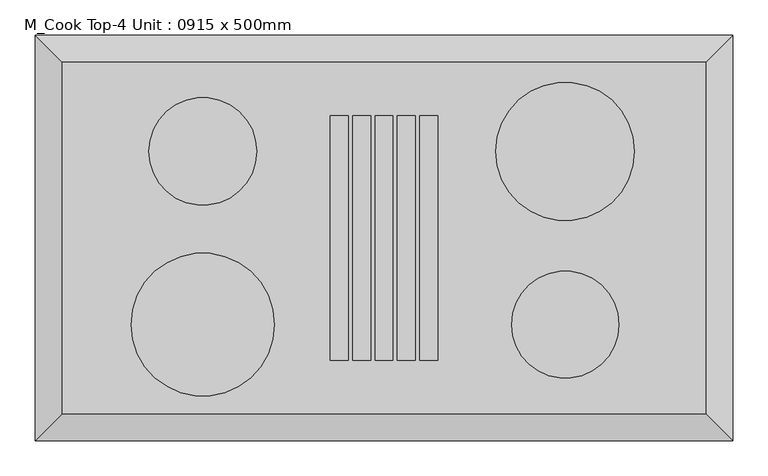
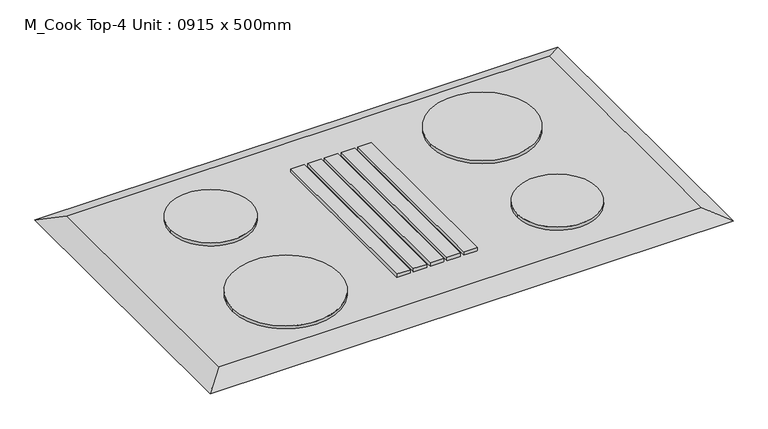
"""IFC4 building model written with IfcOpenShell, lengths in millimetres: proxy geometry, M_Cook Top-4 Unit : 0915 x 500mm."""

from ifc_helpers import new_model, si_unit, point, frame, frame_2d, origin, place, context, project, spatial, polyline, circle_curve, trimmed, segment, composite_curve, outline, extrude, faceted_brep, source, transform, mapped, element, save


def m_cook_top_4_unit_0915_x_500mm_0d6b06ed(model_context):
    return source(origin(), model_context, "Body", "SolidModel", [
        extrude(outline(composite_curve([segment(trimmed(circle_curve(frame_2d((-257.5, 123.0)), 76.5869489), [point((-180.9130511, 123.0))], [point((-334.0869489, 123.0))], False, "CARTESIAN"), True, "CONTINUOUS"), segment(trimmed(circle_curve(frame_2d((-257.5, 123.0)), 76.5869489), [point((-334.0869489, 123.0))], [point((-180.9130511, 123.0))], False, "CARTESIAN"), True, "CONTINUOUS")], self_intersect=False)), frame((0.0, 0.0, 918.0), z_axis=(0.0, 0.0, 1.0), x_axis=(1.0, 0.0, 0.0)), (0.0, 0.0, 1.0), 6.35),
        extrude(outline(composite_curve([segment(trimmed(circle_curve(frame_2d((257.5, 123.0)), 98.4), [point((355.9, 123.0))], [point((159.1, 123.0))], False, "CARTESIAN"), True, "CONTINUOUS"), segment(trimmed(circle_curve(frame_2d((257.5, 123.0)), 98.4), [point((159.1, 123.0))], [point((355.9, 123.0))], False, "CARTESIAN"), True, "CONTINUOUS")], self_intersect=False)), frame((0.0, 0.0, 918.0), z_axis=(0.0, 0.0, 1.0), x_axis=(1.0, 0.0, 0.0)), (0.0, 0.0, 1.0), 6.35),
        extrude(outline(composite_curve([segment(trimmed(circle_curve(frame_2d((257.5, -123.0)), 76.2), [point((333.7, -123.0))], [point((181.3, -123.0))], False, "CARTESIAN"), True, "CONTINUOUS"), segment(trimmed(circle_curve(frame_2d((257.5, -123.0)), 76.2), [point((181.3, -123.0))], [point((333.7, -123.0))], False, "CARTESIAN"), True, "CONTINUOUS")], self_intersect=False)), frame((0.0, 0.0, 918.0), z_axis=(0.0, 0.0, 1.0), x_axis=(1.0, 0.0, 0.0)), (0.0, 0.0, 1.0), 6.35),
        extrude(outline(polyline([(-50.8, 173.8), (-50.8, -173.8), (-76.2, -173.8), (-76.2, 173.8), (-50.8, 173.8)])), frame((0.0, 0.0, 918.0), z_axis=(0.0, 0.0, 1.0), x_axis=(1.0, 0.0, 0.0)), (0.0, 0.0, 1.0), 6.35),
        extrude(outline(polyline([(-19.05, 173.8), (-19.05, -173.8), (-44.45, -173.8), (-44.45, 173.8), (-19.05, 173.8)])), frame((0.0, 0.0, 918.0), z_axis=(0.0, 0.0, 1.0), x_axis=(1.0, 0.0, 0.0)), (0.0, 0.0, 1.0), 6.35),
        extrude(outline(polyline([(12.7, 173.8), (12.7, -173.8), (-12.7, -173.8), (-12.7, 173.8), (12.7, 173.8)])), frame((0.0, 0.0, 918.0), z_axis=(0.0, 0.0, 1.0), x_axis=(1.0, 0.0, 0.0)), (0.0, 0.0, 1.0), 6.35),
        extrude(outline(polyline([(44.45, 173.8), (44.45, -173.8), (19.05, -173.8), (19.05, 173.8), (44.45, 173.8)])), frame((0.0, 0.0, 918.0), z_axis=(0.0, 0.0, 1.0), x_axis=(1.0, 0.0, 0.0)), (0.0, 0.0, 1.0), 6.35),
        extrude(outline(polyline([(76.2, 173.8), (76.2, -173.8), (50.8, -173.8), (50.8, 173.8), (76.2, 173.8)])), frame((0.0, 0.0, 918.0), z_axis=(0.0, 0.0, 1.0), x_axis=(1.0, 0.0, 0.0)), (0.0, 0.0, 1.0), 6.35),
        faceted_brep([(457.5, 250.0, 918.0), (-457.5, 250.0, 918.0), (-457.5, -250.0, 918.0), (457.5, -250.0, 918.0), (495.6, 288.1, 900.0), (495.6, -288.1, 900.0), (-495.6, -288.1, 900.0), (-495.6, 288.1, 900.0)], [[[0, 1, 2, 3]], [[4, 5, 6, 7]], [[4, 7, 1, 0]], [[7, 6, 2, 1]], [[6, 5, 3, 2]], [[5, 4, 0, 3]]]),
        extrude(outline(composite_curve([segment(trimmed(circle_curve(frame_2d((-257.5, -123.0)), 101.6), [point((-155.9, -123.0))], [point((-359.1, -123.0))], False, "CARTESIAN"), True, "CONTINUOUS"), segment(trimmed(circle_curve(frame_2d((-257.5, -123.0)), 101.6), [point((-359.1, -123.0))], [point((-155.9, -123.0))], False, "CARTESIAN"), True, "CONTINUOUS")], self_intersect=False)), frame((0.0, 0.0, 918.0), z_axis=(0.0, 0.0, 1.0), x_axis=(1.0, 0.0, 0.0)), (0.0, 0.0, 1.0), 6.35),
    ])


if __name__ == "__main__":
    model = new_model("IFC4")
    model_context = context("Model", 3, world=origin())
    ifc_project = project(units=[si_unit("LENGTHUNIT", "METRE", prefix="MILLI")], contexts=[model_context])
    site = spatial("IfcSite", under=ifc_project)
    building = spatial("IfcBuilding", under=site)
    placement = place(None, origin())
    m_cook_top_4_unit_0915_x_500mm_shape = m_cook_top_4_unit_0915_x_500mm_0d6b06ed(model_context)
    element("IfcBuildingElementProxy", 1, Name="M_Cook Top-4 Unit : 0915 x 500mm", ObjectType="M_Cook Top-4 Unit : 0915 x 500mm", at=placement, inside=building, context=model_context, shape_type="MappedRepresentation", body=[
        mapped(m_cook_top_4_unit_0915_x_500mm_shape, transform((0.0, 0.0, 0.0), x_axis=(1.0, 0.0, 0.0), y_axis=(0.0, 1.0, 0.0), z_axis=(0.0, 0.0, 1.0))),
    ])
    save(model, "model.ifc")

# Revit data of these elements
# Type "M_Cook Top-4 Unit : 0915 x 500mm"
#   Counter Height = 900 mm
#   Depth = 500 mm
#   Width = 915 mm
#   Burner Material = Steel, Chrome Plated
#   Cooktop Material = Steel, Polished
#   Default Elevation = 0
# Element 1 (IfcBuildingElementProxy, "M_Cook Top-4 Unit : 0915 x 500mm")
#   Materials on its faces: "Steel, Chrome Plated", "Steel, Polished"
# Materials
#   "Steel, Chrome Plated": class "Metal", colour RGB 244 244 244, transparency 0, Description = "Chromiuim plated steel", Cost = 0
#   "Steel, Polished": class "Metal", colour RGB 57 57 57, transparency 0, Description = "Polished steel", Cost = 0
